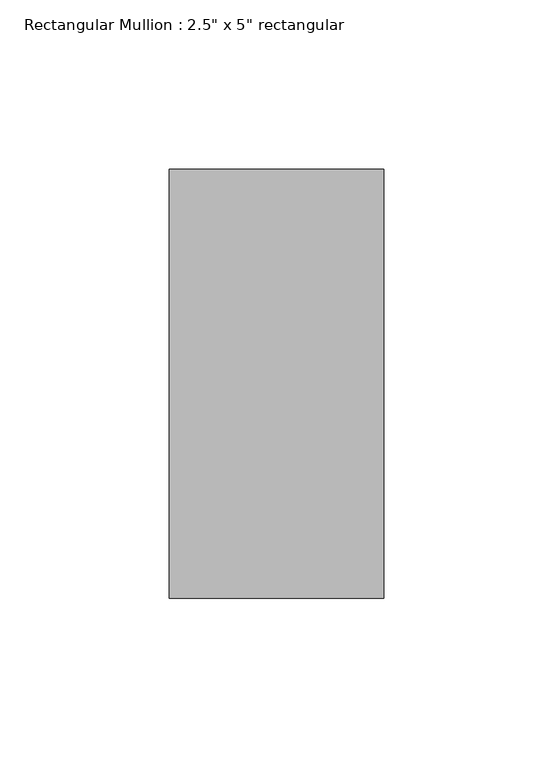
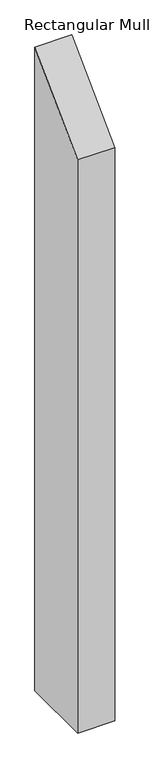
"""IFC4 building model written with IfcOpenShell, lengths in millimetres: member geometry."""

from ifc_helpers import new_model, si_unit, frame, origin, place, context, project, spatial, polyline, outline, extrude, source, transform, mapped, element, save


def member_a361ce75(model_context):
    return source(origin(), model_context, "Body", "SweptSolid", [
        extrude(outline(polyline([(-63.5, -63.5), (63.5, 63.5), (63.5, -1101.969231), (-63.5, -1101.969231), (-63.5, -63.5)])), frame((-31.75, 0.0, 0.0), z_axis=(1.0, 0.0, 0.0), x_axis=(0.0, 1.0, 0.0)), (0.0, 0.0, 1.0), 63.5),
    ])


if __name__ == "__main__":
    model = new_model("IFC4")
    model_context = context("Model", 3, world=origin())
    ifc_project = project(units=[si_unit("LENGTHUNIT", "METRE", prefix="MILLI")], contexts=[model_context])
    site = spatial("IfcSite", under=ifc_project)
    building = spatial("IfcBuilding", under=site)
    placement = place(None, origin())
    member_shape = member_a361ce75(model_context)
    element("IfcMember", 1, ObjectType="Rectangular Mullion : 2.5\" x 5\" rectangular", at=placement, inside=building, context=model_context, shape_type="MappedRepresentation", body=[
        mapped(member_shape, transform((0.0, 0.0, 0.0), x_axis=(1.0, 0.0, 0.0), y_axis=(0.0, 1.0, 0.0), z_axis=(0.0, 0.0, 1.0))),
    ])
    save(model, "model.ifc")

# Revit data of these elements
# Type "Rectangular Mullion : 2.5\" x 5\" rectangular"
#   built-in parameter 1007304 = 0.416667 (stored number, unit not read)
#   built-in parameter 1007301 = 0.104167 (stored number, unit not read)
#   built-in parameter 1007300 = 0.104167 (stored number, unit not read)
# Element 1 (IfcMember, "Rectangular Mullion : 2.5\" x 5\" rectangular")
#   Materials on its faces: "Aluminum"
# Materials
#   "Aluminum": class "Metal", colour RGB 247 247 247, transparency 0, Description = "Aluminum 6061", Cost = 0
